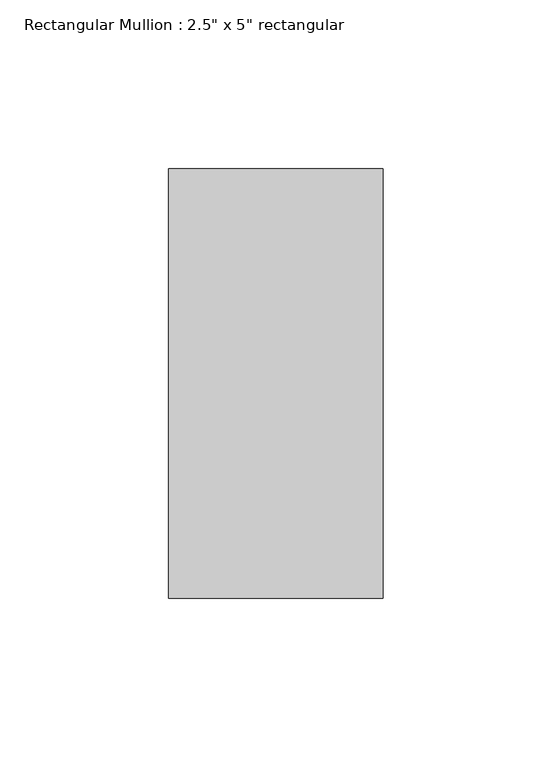
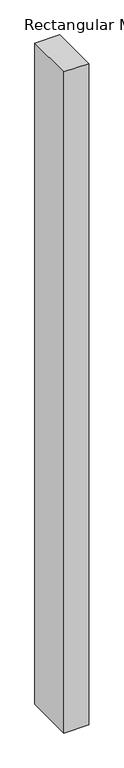
"""IFC4 building model written with IfcOpenShell, lengths in millimetres: member geometry."""

from ifc_helpers import new_model, si_unit, frame, origin, place, context, project, spatial, polyline, outline, extrude, source, transform, mapped, element, save


def member_8182dde8(model_context):
    return source(origin(), model_context, "Body", "SweptSolid", [
        extrude(outline(polyline([(31.75, 63.5), (31.75, -63.5), (-31.75, -63.5), (-31.75, 63.5), (31.75, 63.5)])), frame((0.0, 0.0, -1770.7328538), z_axis=(0.0, 0.0, 1.0), x_axis=(1.0, 0.0, 0.0)), (0.0, 0.0, 1.0), 1770.7328538),
    ])


if __name__ == "__main__":
    model = new_model("IFC4")
    model_context = context("Model", 3, world=origin())
    ifc_project = project(units=[si_unit("LENGTHUNIT", "METRE", prefix="MILLI")], contexts=[model_context])
    site = spatial("IfcSite", under=ifc_project)
    building = spatial("IfcBuilding", under=site)
    placement = place(None, origin())
    member_shape = member_8182dde8(model_context)
    element("IfcMember", 1, ObjectType="Rectangular Mullion : 2.5\" x 5\" rectangular", at=placement, inside=building, context=model_context, shape_type="MappedRepresentation", body=[
        mapped(member_shape, transform((0.0, 0.0, 0.0), x_axis=(1.0, 0.0, 0.0), y_axis=(0.0, 1.0, 0.0), z_axis=(0.0, 0.0, 1.0))),
    ])
    save(model, "model.ifc")

# Revit data of these elements
# Type "Rectangular Mullion : 2.5\" x 5\" rectangular"
#   built-in parameter 1007304 = 0.416667 (stored number, unit not read)
#   built-in parameter 1007301 = 0.104167 (stored number, unit not read)
#   built-in parameter 1007300 = 0.104167 (stored number, unit not read)
# Element 1 (IfcMember, "Rectangular Mullion : 2.5\" x 5\" rectangular")
#   Materials on its faces: "Aluminum"
# Materials
#   "Aluminum": class "Metal", colour RGB 247 247 247, transparency 0, Description = "Aluminum 6061", Cost = 0
